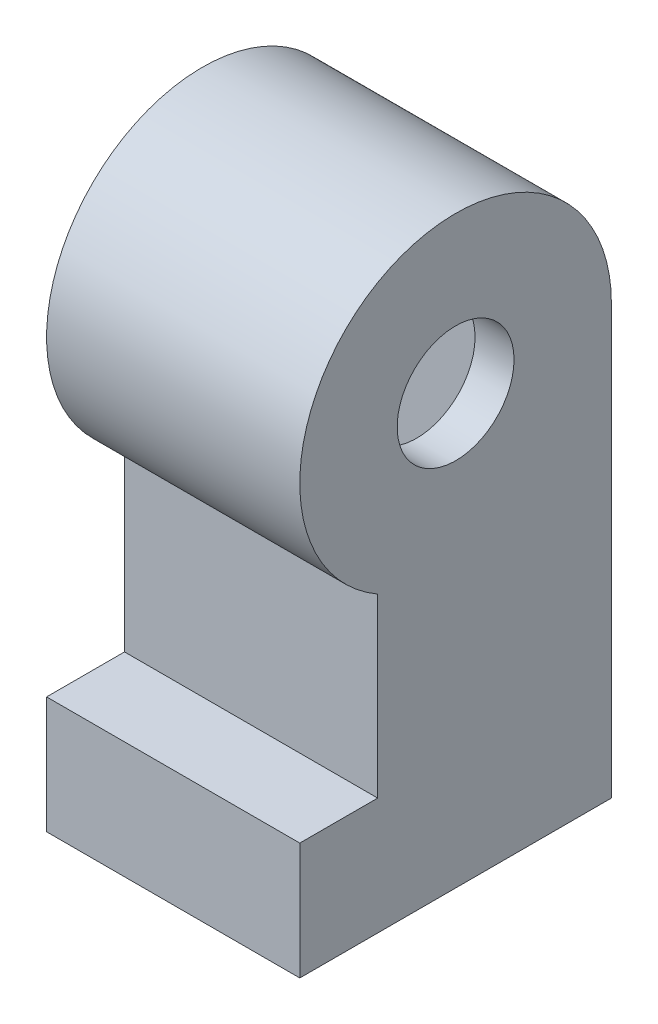
SolidWorks part; units mm, degrees
material "Plain Carbon Steel"
ref_plane "Front Plane" through (0, 0, 0) normal (0, 0, 1) x (1, 0, 0)
ref_plane "Top Plane" through (0, 0, 0) normal (0, 1, 0) x (1, 0, 0)
ref_plane "Right Plane" through (0, 0, 0) normal (1, 0, 0) x (0, 0, -1)
sketch "Leg Profile Sketch" plane through (0, 0, 0) normal (1, 0, 0) x (0, 0, -1)
  line L0 (4, 0) -> (4, -11)
  line L1 (4, -11) -> (-4, -11)
  line L2 (-4, -11) -> (-4, -8)
  line L3 (-4, -8) -> (-2, -8)
  line L4 (-2, -8) -> (-2, -3.4641)
  arc A0 (4, 0) -> (-2, -3.4641) centre (0, 0) ccw
  dimension "D1" = 8
  dimension "D2" = 11
  dimension "D3" = 8
  dimension "D4" = 3
  dimension "D5" = 2
extrude "Leg Body" add sketch "Leg Profile Sketch" along normal blind 6.5
shell "Leg Shell 1mm" thickness 1
sketch "Hip Pin Hole Sketch" plane through (6.5, 0, 0) normal (1, 0, 0) x (0, 0, -1)
  circle A0 centre (0, 0) radius 1.5
  dimension "D1" = 3
extrude "Hip Pin Hole" cut sketch "Hip Pin Hole Sketch" against normal up to next
